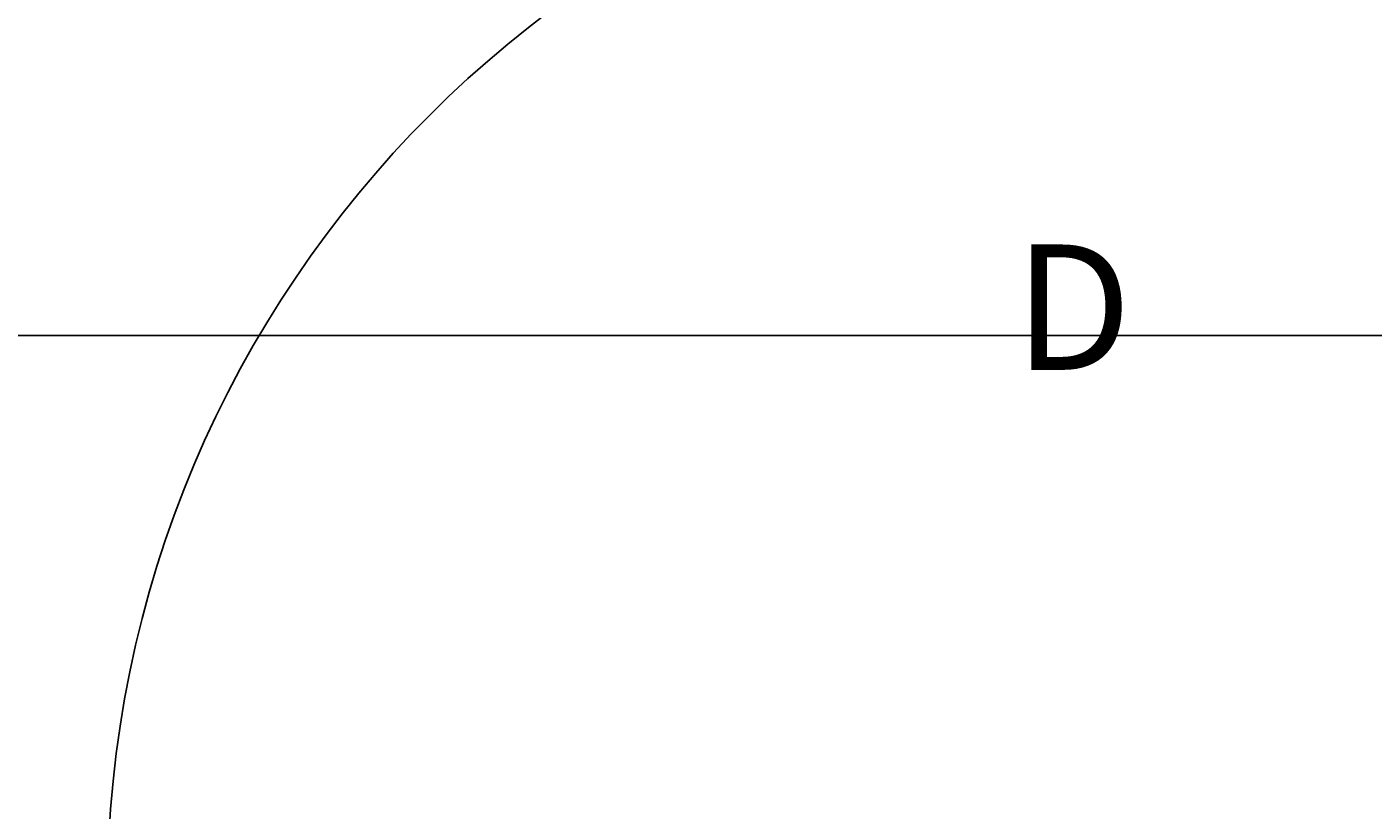
# Model space of a CAD drawing. Units: inches. Extents: x 1998 to 2588, y 1139 to 1977.
# Tile 9 of 134: x 2075 to 2115, y 1599 to 1622. Entities that reach past the tile are written whole.
import ezdxf

# ---------------------------------------------------------------- set-up
doc = ezdxf.new("R2010")
doc.units = ezdxf.units.IN
for name, color, linetype, lineweight in [('A-ANNO-DIMS', 2, 'Continuous', 18), ('A-DOOR-IDEN', 7, 'Continuous', 18), ('DOOR', 52, 'Continuous', 25)]:
    doc.layers.add(name, color=color, linetype=linetype, lineweight=lineweight)
doc.styles.get("Standard").update_dxf_attribs({"font": 'arial.ttf'})
doc.dimstyles.get("Standard").update_dxf_attribs({"dimtxt": 0.18, "dimasz": 0.18, "dimexe": 0.18, "dimexo": 0.0625, "dimgap": 0.09, "dimtad": 0, "dimtih": 1, "dimtoh": 1, "dimdec": 4, "dimzin": 0, "dimdsep": 46, "dimtxsty": 'Standard', "dimcen": 0.09, "dimadec": 0, "dimazin": 0, "dimtfac": 1, "dimtdec": 4, "dimtofl": 0, "dimtmove": 0, "dimatfit": 3, "dimfxl": 1, "dimtolj": 1, "dimtzin": 0, "dimarcsym": 0})

# ---------------------------------------------------------------- blocks, each defined once
blk = doc.blocks.new('*U2')
for p, q in [((0, 0), (0, -6)), ((40, 0), (40, -6))]:
    blk.add_line(p, q)
blk.add_lwpolyline([(0, 0), (0, 40), (1.75, 40), (1.75, 0)], close=True)
blk.add_arc((0, 0), 40, 0, 90)
blk = doc.blocks.new('*D30')
at = {"layer": 'A-ANNO-DIMS', "color": 0, "lineweight": -2, "transparency": 16777216}
for p, q in [((2407.91, 1636.732), (1997.843, 1636.732)), ((1998.023, 1636.552), (1998.023, 1615.913)), ((1998.023, 1594.912), (1998.023, 1615.552)), ((2407.91, 1594.732), (1997.843, 1594.732))]:
    blk.add_line(p, q, dxfattribs=at)
at = {"layer": 'A-ANNO-DIMS', "color": 0, "transparency": 16777216}
for points in [[(1997.993, 1636.552), (1998.053, 1636.552), (1998.023, 1636.732)], [(1997.993, 1594.912), (1998.053, 1594.912), (1998.023, 1594.732)]]:
    blk.add_solid(points, dxfattribs=at)
at = {"layer": 'Defpoints', "color": 0, "transparency": 16777216}
for p in [(1998.023, 1636.732), (2407.973, 1636.732), (2407.973, 1594.732)]:
    blk.add_point(p, dxfattribs=at)
at = {"layer": 'A-ANNO-DIMS', "color": 0, "transparency": 16777216, "insert": (1998.023, 1615.732), "char_height": 0.18, "attachment_point": 5}
blk.add_mtext('\\A1;42', dxfattribs=at)
blk = doc.blocks.new('*D35')
at = {"layer": 'A-ANNO-DIMS', "color": 0, "lineweight": -2, "transparency": 16777216}
for p, q in [((2148.392, 1612.732), (1997.843, 1612.732)), ((1998.023, 1612.552), (1998.023, 1600.913)), ((1998.023, 1588.912), (1998.023, 1600.552)), ((2148.392, 1588.732), (1997.843, 1588.732))]:
    blk.add_line(p, q, dxfattribs=at)
at = {"layer": 'A-ANNO-DIMS', "color": 0, "transparency": 16777216}
for points in [[(1997.993, 1612.552), (1998.053, 1612.552), (1998.023, 1612.732)], [(1997.993, 1588.912), (1998.053, 1588.912), (1998.023, 1588.732)]]:
    blk.add_solid(points, dxfattribs=at)
at = {"layer": 'Defpoints', "color": 0, "transparency": 16777216}
for p in [(1998.023, 1612.732), (2148.455, 1612.732), (2148.455, 1588.732)]:
    blk.add_point(p, dxfattribs=at)
at = {"layer": 'A-ANNO-DIMS', "color": 0, "transparency": 16777216, "insert": (1998.023, 1600.732), "char_height": 0.18, "attachment_point": 5}
blk.add_mtext('\\A1;24', dxfattribs=at)
blk = doc.blocks.new('*D38')
at = {"layer": 'A-ANNO-DIMS', "color": 0, "lineweight": -2, "transparency": 16777216}
for p, q in [((2197.387, 1663.247), (1997.843, 1663.247)), ((1998.023, 1663.067), (1998.023, 1638.171)), ((1998.023, 1612.912), (1998.023, 1637.808)), ((2197.387, 1612.732), (1997.843, 1612.732))]:
    blk.add_line(p, q, dxfattribs=at)
at = {"layer": 'A-ANNO-DIMS', "color": 0, "transparency": 16777216}
for points in [[(1997.993, 1663.067), (1998.053, 1663.067), (1998.023, 1663.247)], [(1997.993, 1612.912), (1998.053, 1612.912), (1998.023, 1612.732)]]:
    blk.add_solid(points, dxfattribs=at)
at = {"layer": 'Defpoints', "color": 0, "transparency": 16777216}
for p in [(1998.023, 1663.247), (2197.45, 1663.247), (2197.45, 1612.732)]:
    blk.add_point(p, dxfattribs=at)
at = {"layer": 'A-ANNO-DIMS', "color": 0, "transparency": 16777216, "insert": (1998.023, 1637.99), "char_height": 0.18, "attachment_point": 5}
blk.add_mtext('\\A1;50.51', dxfattribs=at)

msp = doc.modelspace()

# ---------------------------------------------------------------- block references
at = {"layer": 'DOOR', "xscale": 0.8119355758402486, "yscale": 0.8119355758402486, "zscale": 0.8119355758402486, "rotation": 90.00000000000003}
msp.add_blockref('*U2', (2110.1012, 1596.2642), dxfattribs=at)

# ---------------------------------------------------------------- texts
at = {"layer": 'A-DOOR-IDEN', "insert": (2104.3803, 1615.413), "char_height": 3.6988, "attachment_point": 1}
msp.add_mtext_dynamic_manual_height_columns('D', width=110.572713, gutter_width=18.4938, heights=[0], dxfattribs=at)

# ---------------------------------------------------------------- dimensions: what is measured, and where the dimension line sits
at = {"layer": 'A-ANNO-DIMS'}
for base, p1, p2, override, picture, middle in [((1998.0229, 1663.2466), (2197.4499, 1612.7324), (2197.4499, 1663.2466), {"dimdec": 2, "dimlfac": 1, "dimrnd": 0, "dimzin": 0, "dimdsep": 46, "dimlunit": 2}, '*D38', (1998.0229, 1637.9895)), ((1998.0229, 1636.7324), (2407.9729, 1594.7324), (2407.9729, 1636.7324), {"dimdec": 0, "dimlfac": 1, "dimrnd": 0, "dimzin": 0, "dimdsep": 46, "dimlunit": 2}, '*D30', (1998.0229, 1615.7324)), ((1998.0229, 1612.7324), (2148.4548, 1588.7324), (2148.4548, 1612.7324), {"dimdec": 0, "dimlfac": 1, "dimrnd": 0, "dimzin": 0, "dimdsep": 46, "dimlunit": 2}, '*D35', (1998.0229, 1600.7324))]:
    dim = msp.add_linear_dim(base=base, p1=p1, p2=p2, angle=90, dimstyle='Standard', override=override, dxfattribs=at)
    dim.commit()
    dim.dimension.update_dxf_attribs({"geometry": picture, "text_midpoint": middle})

doc.saveas('drawing.dxf')
